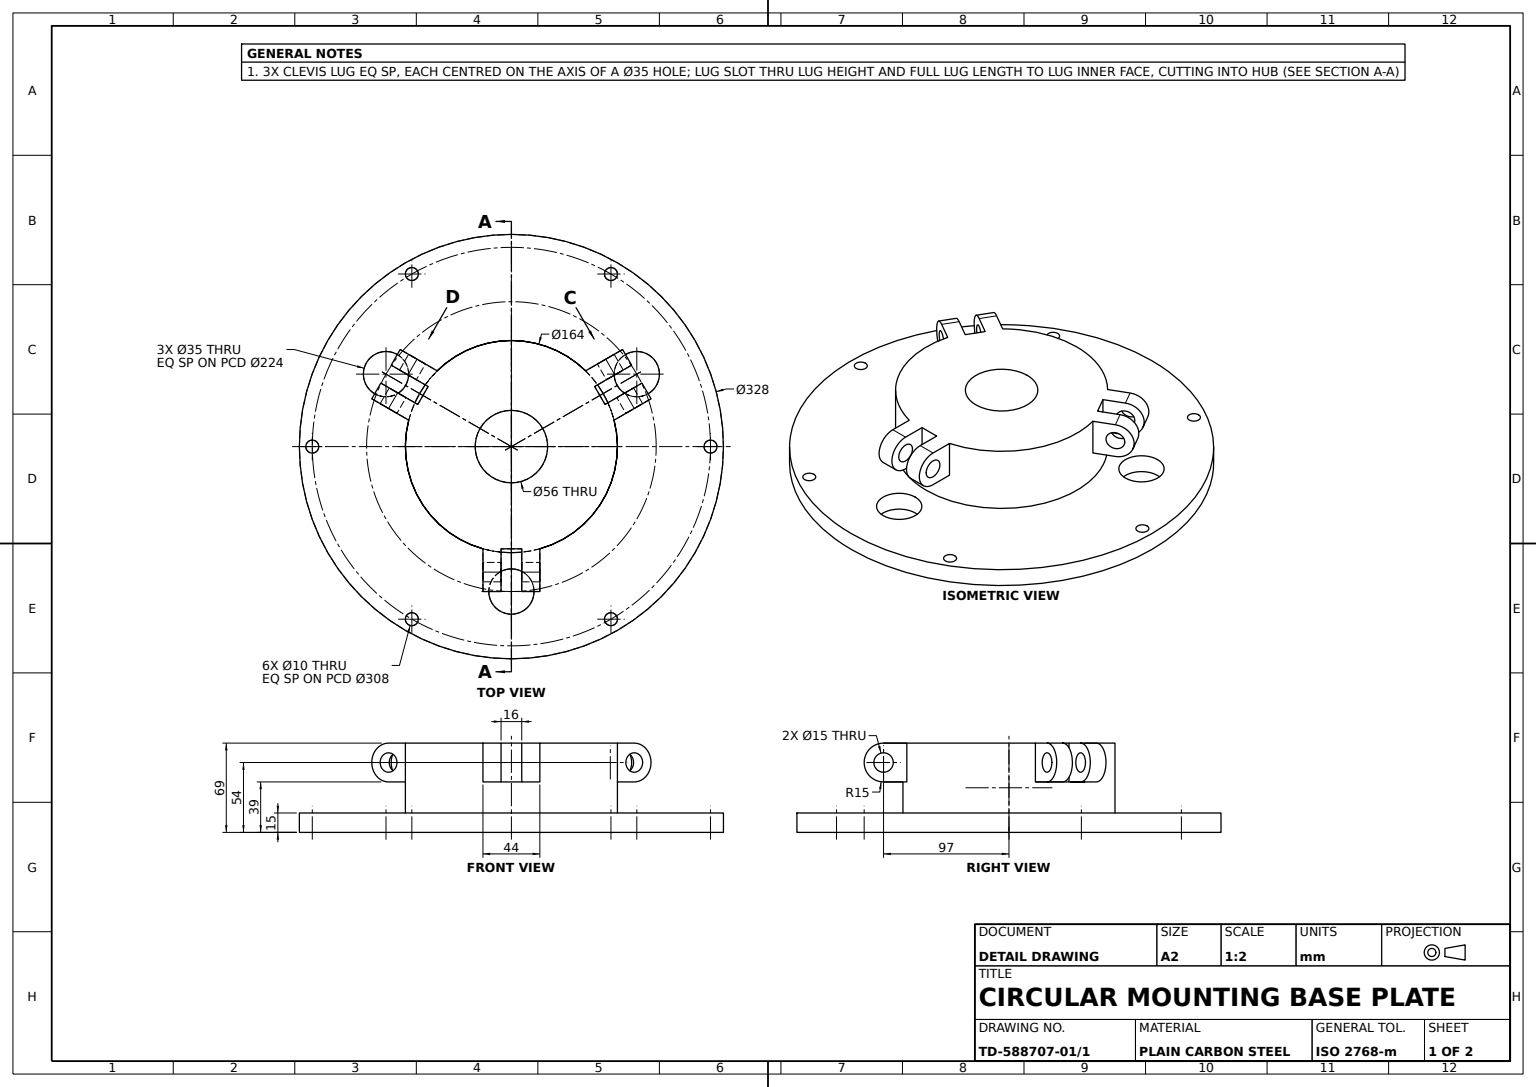
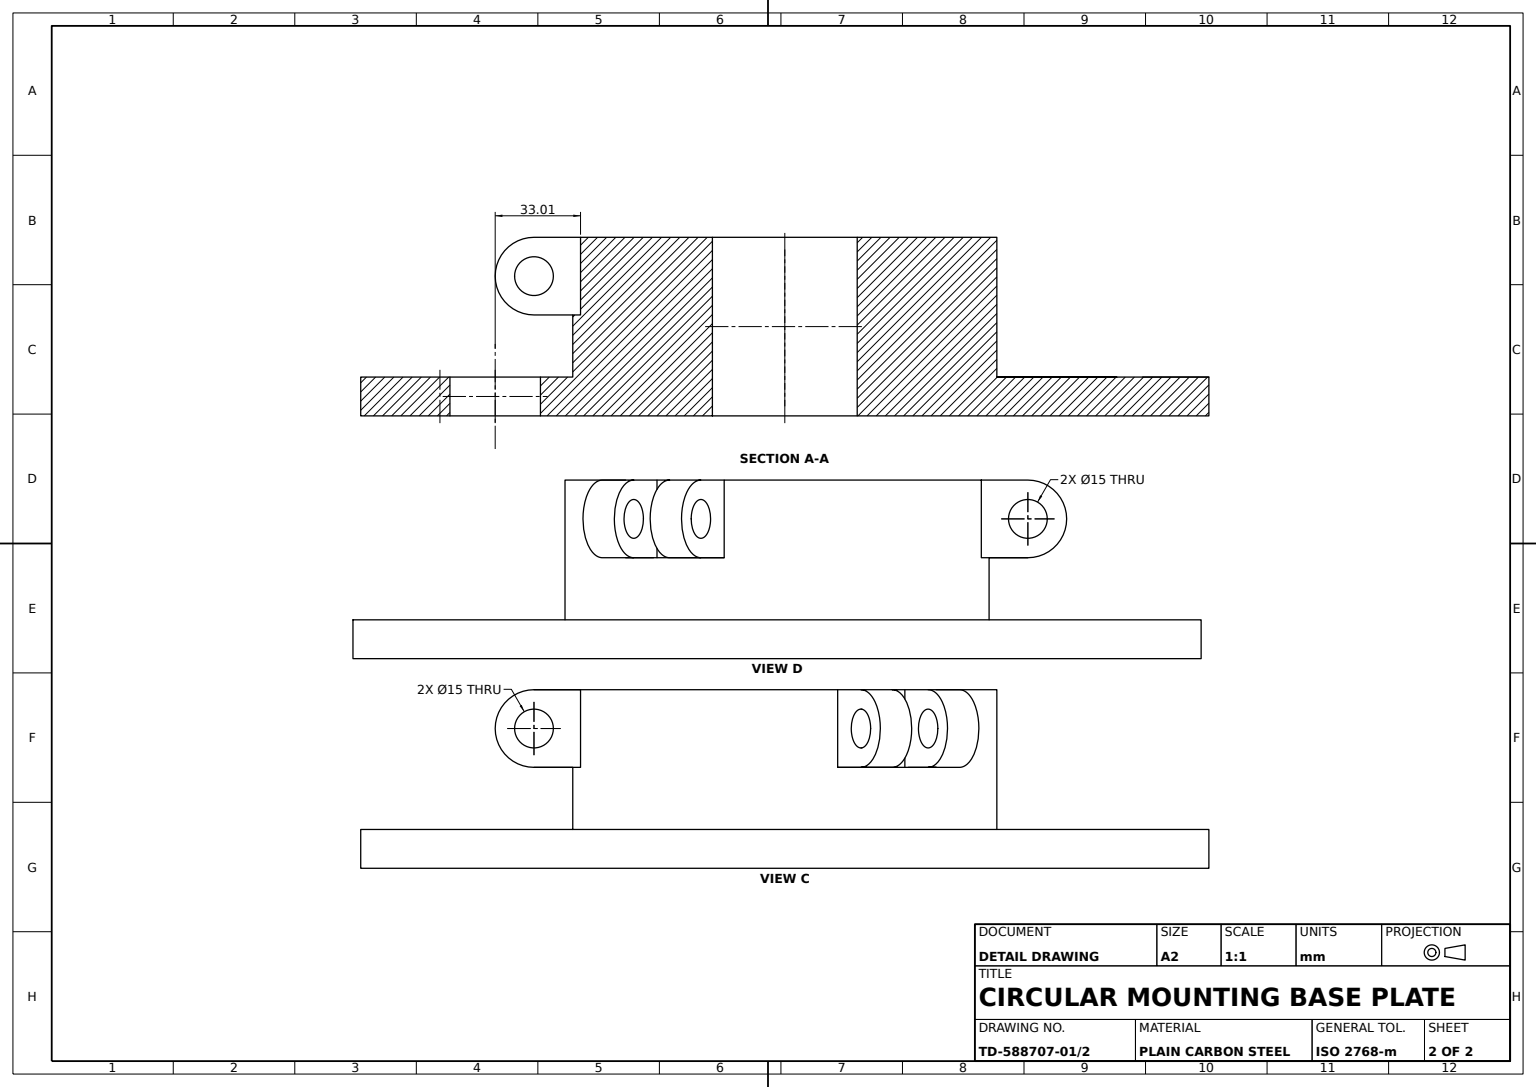
SolidWorks part; units mm, degrees
material "Plain Carbon Steel"
ref_plane "Front Plane" through (0, 0, 0) normal (0, 0, 1) x (1, 0, 0)
ref_plane "Top Plane" through (0, 0, 0) normal (0, 1, 0) x (1, 0, 0)
ref_plane "Right Plane" through (0, 0, 0) normal (1, 0, 0) x (0, 0, -1)
sketch "Base Disc Sketch Ø328" plane through (0, 0, 0) normal (0, 1, 0) x (1, 0, 0)
  circle A0 centre (0, 0) radius 164
  dimension "D1" = 328
extrude "Base Disc Ø328x15" add sketch "Base Disc Sketch Ø328" along normal blind 15
sketch "Hub Sketch Ø164" plane through (0, 15, 0) normal (0, 1, 0) x (1, 0, 0)
  circle A0 centre (0, 0) radius 82
  dimension "D1" = 164
extrude "Hub Ø164x54" add sketch "Hub Sketch Ø164" along normal blind 54
sketch "Centre Bore Sketch Ø56" plane through (0, 69, 0) normal (0, 1, 0) x (1, 0, 0)
  circle A0 centre (0, 0) radius 28
  dimension "D1" = 56
extrude "Centre Bore Ø56" cut sketch "Centre Bore Sketch Ø56" against normal through all
sketch "Clevis Reference Line Sketch" plane through (0, 69, 0) normal (0, 1, 0) x (1, 0, 0)
  line L0 (0, 0) -> (0, -82) construction
  circle A0 centre (0, 0) radius 82 construction
ref_plane "Plane2" through (0, 0, 0) normal (1, 0, 0) x (0, 0, -1)
sketch "Clevis Lug Profile Sketch" plane through (0, 0, 0) normal (1, 0, 0) x (0, 0, -1)
  line L0 (-82, 69) -> (-82, 39) construction
  line L1 (-82, 69) -> (-82, 15) construction
  line L2 (-97, 69) -> (-69.4082, 69)
  line L4 (0, 69) -> (-82, 69) construction
  line L5 (-69.4082, 69) -> (-69.4082, 39)
  line L6 (-69.4082, 39) -> (-97, 39)
  circle A0 centre (-97, 54) radius 7.5
  arc A1 (-97, 69) -> (-97, 39) centre (-97, 54) ccw
  dimension "D1" = 30
  dimension "D2" = 15
  dimension "D3" = 97
  dimension "D4" = 12.5918
extrude "Clevis Lug" add sketch "Clevis Lug Profile Sketch" along normal mid plane 44
ref_plane "Plane3" through (0, 69, 0) normal (0, 1, 0) x (1, 0, 0)
sketch "Clevis Slot Profile Sketch" plane through (0, 69, 0) normal (0, 1, 0) x (1, 0, 0)
  line L0 (0, -82) -> (0, -112) construction
  line L1 (-22, -112) -> (22, -112) construction
  line L2 (0, -112) -> (-8, -112)
  line L3 (-8, -112) -> (-8, -78.9937)
  line L4 (-8, -78.9937) -> (8, -78.9937)
  line L5 (8, -78.9937) -> (8, -112)
  line L6 (8, -112) -> (0, -112)
  dimension "D1" = 8
  dimension "D2" = 33.0063
extrude "Clevis Slot 30" cut sketch "Clevis Slot Profile Sketch" against normal blind 30
pattern_circular "Clevis Lug Pattern 3x" count 3 over 360 about axis through (0, 0, 0) along (0, 1, 0) of "Clevis Slot 30", "Clevis Lug"
sketch "Large Hole Sketch Ø35" plane through (0, 15, 0) normal (0, 1, 0) x (1, 0, 0)
  circle A0 centre (0, -112) radius 17.5
  circle A1 centre (0, 0) radius 82 construction
  dimension "D1" = 35
  dimension "D2" = 112
  dimension "D3" = 112
extrude "Large Hole Ø35" cut sketch "Large Hole Sketch Ø35" against normal through all
pattern_circular "Large Hole Pattern 3xØ35" count 3 over 360 about axis through (0, 0, 0) along (0, 1, 0) of "Large Hole Ø35"
sketch "Mounting Hole Sketch Ø10" plane through (0, 69, 0) normal (0, 1, 0) x (1, 0, 0)
  line L0 (0, -94.5) -> (0, -129.5) construction
  line L1 (-17.5, -112) -> (17.5, -112) construction
  line L2 (-22, -112) -> (-8, -112) construction
  line L4 (22, -97) -> (8, -97) construction
  circle A0 centre (-154, 0) radius 5
  circle A1 centre (0, -112) radius 17.5 construction
  point P11 (0, -112)
  dimension "D1" = 10
  dimension "D2" = 154
  dimension "D3" = 97
extrude "Mounting Hole Ø10" cut sketch "Mounting Hole Sketch Ø10" against normal through all
pattern_circular "Mounting Hole Pattern 6xØ10" count 6 over 360 about axis through (0, 0, 0) along (0, 1, 0) of "Mounting Hole Ø10"
